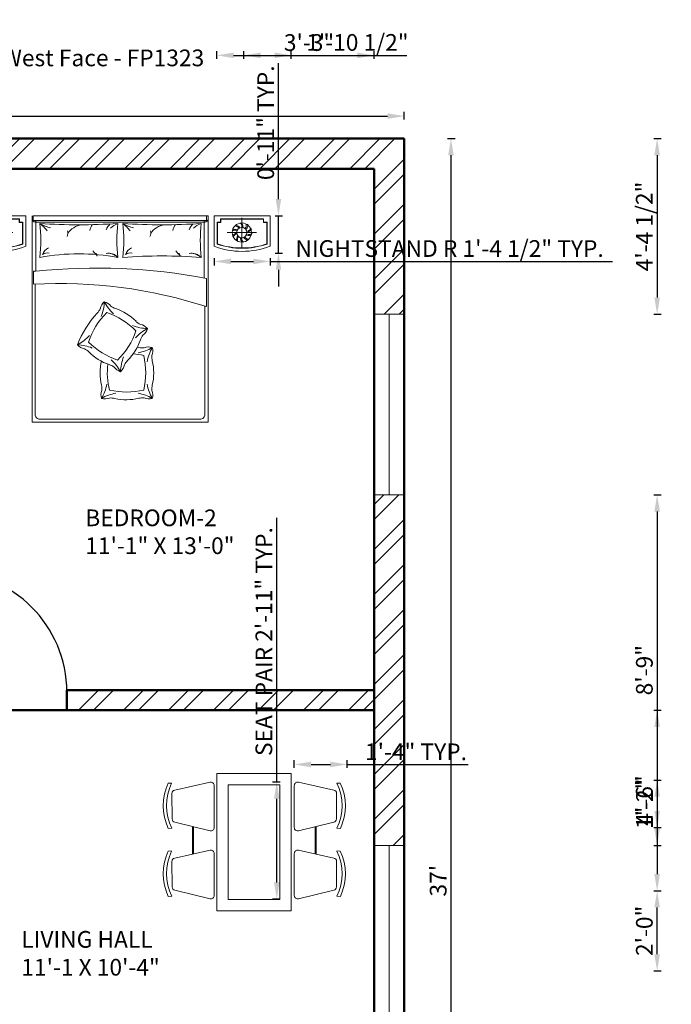
# Model space of a CAD drawing. Units: inches. Extents: x -83 to 371, y -457 to 76.
# Tile 4 of 4: x 176 to 371, y -243 to 51. Entities that reach past the tile are written whole.
import ezdxf

# ---------------------------------------------------------------- set-up
doc = ezdxf.new("R2010")
doc.units = ezdxf.units.IN
for name, color, linetype, lineweight in [('A-ANNO-DIMS', 2, 'Continuous', 18), ('A-ANNO-TEXT', 7, 'Continuous', 25), ('A-AREA-IDEN', 7, 'Continuous', 25), ('A-DOOR', 3, 'Continuous', 25), ('A-GLAZ', 4, 'Continuous', 18), ('A-WALL', 7, 'Continuous', 50), ('A-WALL-PATT', 252, 'Continuous', 13), ('furn', 28, 'Continuous', 18)]:
    doc.layers.add(name, color=color, linetype=linetype, lineweight=lineweight)
doc.styles.get("Standard").update_dxf_attribs({"font": 'arial.ttf'})
doc.dimstyles.new('ISO-25', dxfattribs={"dimtxt": 5, "dimasz": 5, "dimexe": 1.25, "dimexo": 0.625, "dimtad": 1, "dimlunit": 3, "dimtxsty": 'Standard', "dimcen": 2.5, "dimadec": 0, "dimazin": 0, "dimtfac": 1, "dimtmove": 0, "dimatfit": 3, "dimfxl": 1, "dimfxlon": 1, "dimarcsym": 0})

# ---------------------------------------------------------------- blocks, each defined once
blk = doc.blocks.new('*U4')
for p, q in [((0, 0), (0, -6)), ((40, 0), (40, -6))]:
    blk.add_line(p, q)
blk.add_lwpolyline([(0, 0), (0, 40), (1.75, 40), (1.75, 0)], close=True)
blk.add_arc((0, 0), 40, 0, 90)
blk = doc.blocks.new('*D8')
at = {"layer": 'A-ANNO-DIMS', "color": 0, "lineweight": -2, "transparency": 16777216}
for p, q in [((2.97, 21.4), (2.97, 23.65)), ((290.97, 21.4), (290.97, 23.65)), ((7.97, 22.4), (285.97, 22.4))]:
    blk.add_line(p, q, dxfattribs=at)
at = {"layer": 'A-ANNO-DIMS', "color": 0, "transparency": 16777216}
for points in [[(7.97, 23.23), (7.97, 21.56), (2.97, 22.4)], [(285.97, 23.23), (285.97, 21.56), (290.97, 22.4)]]:
    blk.add_solid(points, dxfattribs=at)
at = {"layer": 'Defpoints', "color": 0, "transparency": 16777216}
for p in [(290.97, 22.4), (2.97, 15.68), (290.97, 15.68)]:
    blk.add_point(p, dxfattribs=at)
at = {"layer": 'A-ANNO-DIMS', "color": 0, "transparency": 16777216, "insert": (146.97, 25.53), "char_height": 5, "attachment_point": 5}
blk.add_mtext("24'", dxfattribs=at)
blk = doc.blocks.new('*D9')
at = {"layer": 'A-ANNO-DIMS', "color": 0, "lineweight": -2, "transparency": 16777216}
for p, q in [((303.95, 15.68), (306.2, 15.68)), ((304.95, 10.68), (304.95, -423.32)), ((303.95, -428.32), (306.2, -428.32))]:
    blk.add_line(p, q, dxfattribs=at)
at = {"layer": 'A-ANNO-DIMS', "color": 0, "transparency": 16777216}
for points in [[(304.12, 10.68), (305.78, 10.68), (304.95, 15.68)], [(304.12, -423.32), (305.78, -423.32), (304.95, -428.32)]]:
    blk.add_solid(points, dxfattribs=at)
at = {"layer": 'Defpoints', "color": 0, "transparency": 16777216}
for p in [(295.93, 15.68), (290.97, -428.32), (304.95, -428.32)]:
    blk.add_point(p, dxfattribs=at)
at = {"layer": 'A-ANNO-DIMS', "color": 0, "transparency": 16777216, "insert": (301.77, -206.32), "char_height": 5, "attachment_point": 5, "rotation": 90}
blk.add_mtext("37'", dxfattribs=at)
blk = doc.blocks.new('BED-DOUBLE')
for p, q in [((0.91, 59.91), (51.75, 59.91)), ((1.17, 60.37), (1.17, 45.16)), ((51.46, 60.37), (51.46, 43.19))]:
    blk.add_line(p, q)
for points in [[(0, 61.8), (0, 0), (52.66, 0), (52.66, 61.8)], [(52.17, 61.8), (52.17, 60.37), (0.3, 60.37), (0.3, 61.8), (52.66, 61.8)]]:
    blk.add_lwpolyline(points)
for points in [[(2.33, 49.32, 0.058596), (2.33, 59.5, 0.036889), (25.64, 59.5, 0.052163), (25.64, 49.32, 0.093111)], [(27.16, 49.32, 0.058596), (27.16, 59.5, 0.036648), (50.62, 59.5, 0.052163), (50.62, 49.32, 0.036967)], [(0.46, 45.16), (1.17, 45.16, -0.072944), (52.17, 43.04), (52.17, 34.6, 0.092568), (0.46, 41.29)]]:
    blk.add_lwpolyline(points, format="xyb", close=True)
for points in [[(0.91, 41.32), (0.91, 2.43, 0.414214), (2.43, 0.91), (50.23, 0.91, 0.414214), (51.75, 2.43), (51.75, 34.75)], [(20.68, 31.62, 0.091296), (21.61, 36.08, 0.091296), (24.41, 32.49, 0.091296)], [(16.91, 24, 0.111006), (25.6, 18.59, 0.119549), (31.09, 27.39, 0.107813), (22.42, 32.82)], [(22.37, 32.81, 0.121865), (16.91, 24, 0.121865)], [(26.47, 15.11, 0.159461), (27.65, 17.2, -0.076283), (28.59, 18.51, 0.115075), (32.41, 24.64, -0.076283), (33.17, 26.05, 0.159461), (34.52, 28.03)], [(30.07, 28.97, 0.091296), (34.52, 28.03, 0.091296), (30.93, 25.24, 0.091296)], [(18.01, 22.22, 0.091296), (13.56, 23.16, 0.091296), (17.15, 25.96, 0.091296)], [(31.71, 20.79, 0.091296), (35.99, 22.35, 0.091296), (34.42, 18.08, 0.091296)], [(35.99, 7.13, 0.159461), (35.88, 9.53, -0.076283), (35.99, 11.13, 0.115075), (35.99, 18.36, -0.076283), (35.88, 19.96, 0.159461), (35.99, 22.35)], [(23.17, 9.62, 0.111006), (33.41, 9.63, 0.119549), (33.41, 19.99, 0.033212), (30.26, 20.47)], [(27.4, 19.57, 0.091296), (26.47, 15.11, 0.091296), (23.67, 18.7)], [(25.05, 8.69, 0.091296), (20.77, 7.13, 0.091296), (22.34, 11.41, 0.091296)], [(34.42, 11.41, 0.091296), (35.99, 7.13, 0.091296), (31.71, 8.69)]]:
    blk.add_lwpolyline(points, format="xyb")
for centre, radius, start, end in [((0.91, 60.83), 0.913, 180, 270), ((7.74, 68), 10.08, 237.5379, 257.5233), ((-5.29, 49.98), 12.19, 36.4935, 51.2792), ((15.48, 53.46), 5.64, 96.6849, 148.3182), ((21.18, 56.67), 3.96, 141.8174, 169.8987), ((26.19, 56.11), 4.26, 130.5354, 160.3558), ((28.84, 52.52), 7.67, 114.6457, 134.1585), ((19.53, 49.98), 12.19, 36.4935, 51.2792), ((32.57, 68), 10.08, 237.5379, 257.5233), ((40.3, 53.46), 5.64, 96.6849, 148.3182), ((46.01, 56.67), 3.96, 141.8174, 169.8987), ((51.01, 56.11), 4.26, 130.5354, 160.3558), ((53.67, 52.52), 7.67, 114.6457, 134.1585), ((51.75, 60.83), 0.913, 270, 0), ((8.15, 56.6), 2.53, 335.8927, 16.1192), ((32.98, 56.6), 2.53, 335.8927, 16.1192), ((6.34, 49.09), 3.38, 114.2916, 160.9896), ((4.59, 48.38), 2.31, 76.4823, 128.5563), ((9.19, 42.25), 12.71, 36.2085, 45.0849), ((18.6, 49.75), 0.853, 353.7543, 77.2187), ((22.67, 46.41), 4.16, 44.406, 96.8342), ((23.45, 47.86), 2.64, 33.6349, 90.8456), ((31.17, 49.09), 3.38, 114.2916, 160.9896), ((29.41, 48.38), 2.31, 76.4823, 128.5563), ((34.02, 42.25), 12.71, 36.2085, 45.0849), ((43.42, 49.75), 0.853, 353.7543, 77.2187), ((47.5, 46.41), 4.16, 44.406, 96.8342), ((48.27, 47.86), 2.64, 33.6349, 90.8456), ((24.21, 33.23), 3.86, 132.4658, 168.7065), ((20.58, 32.5), 3.72, 37.2937, 74.0973), ((44.41, 10.55), 33.33, 138.3818, 157.7644), ((15.72, 36.39), 5.29, 315.5854, 333.0343), ((26.71, 38.99), 5.29, 233.2983, 250.7472), ((19.89, 18.93), 15.91, 45.1307, 71.3884), ((34.79, 33.99), 5.29, 225.7718, 243.2208), ((31.77, 25.77), 3.56, 39.4726, 79.6505), ((16.39, 25.78), 3.86, 222.6522, 258.8929), ((13.27, 17.27), 5.29, 45.7718, 63.2208), ((28.18, 32.33), 15.91, 225.1307, 251.3884), ((28.38, 6.89), 15.91, 77.0576, 78.7033), ((33.07, 27.55), 5.29, 257.6988, 275.1477), ((34.85, 18.98), 3.56, 71.3996, 111.5774), ((36.26, 14.74), 15.91, 166.8711, 193.1289), ((44.1, 14.85), 21.58, 173.1956, 194.0284), ((21.36, 12.27), 5.29, 53.2983, 70.7472), ((27.96, 19.27), 4.41, 218.7754, 250.3571), ((24.48, 8.17), 3.86, 159.3666, 195.6073), ((15.61, 9.99), 5.29, 355.0387, 12.4877), ((21.79, 10.85), 3.86, 254.5791, 290.8198), ((23.64, 1.98), 5.29, 77.6988, 95.1477), ((28.33, 22.65), 15.91, 257.0576, 283.3153), ((33.15, 2.01), 5.29, 85.2252, 102.6741), ((35.05, 11.45), 4.41, 250.7023, 282.284)]:
    blk.add_arc(centre, radius, start, end)
blk = doc.blocks.new('NIGHTSTAND-L')
for p, q in [((8.46, 1.22), (8.46, 10)), ((4.07, 5.61), (12.85, 5.61))]:
    blk.add_line(p, q)
blk.add_lwpolyline([(0, 1.52), (0, 10.65), (16.74, 10.65), (16.74, 1.52, -0.181818)], format="xyb", close=True)
for points in [[(1.92, 9.74), (1.92, 8.74), (0.91, 8.74)], [(2.01, 9.74), (2.01, 8.65), (0.91, 8.65)], [(1.92, 9.74), (14.83, 9.74)], [(1.92, 9.65), (14.83, 9.65)], [(14.73, 9.74), (14.73, 8.65), (15.83, 8.65)], [(14.83, 9.74), (14.83, 8.74), (15.83, 8.74)]]:
    blk.add_lwpolyline(points)
for points in [[(15.83, 8.74), (15.83, 2.16, -0.167087), (0.91, 2.16), (0.91, 8.74)], [(15.74, 8.74), (15.74, 2.22, -0.165559), (1, 2.22), (1, 8.74)]]:
    blk.add_lwpolyline(points, format="xyb")
for radius in [2.87, 1.55]:
    blk.add_circle((8.46, 5.61), radius)
for centre, radius, start, end in [((7.4, 7.5), 1.84, 208.17, 254.4897), ((7.28, 7.36), 1.41, 196.3002, 256.538), ((8.71, 7.76), 1.84, 172.17, 218.4897), ((8.53, 7.72), 1.41, 160.3002, 220.538), ((9.93, 7.2), 1.84, 136.17, 182.4897), ((9.76, 7.27), 1.41, 124.3002, 184.538), ((10.58, 6.04), 1.84, 100.17, 146.4897), ((10.49, 6.19), 1.41, 88.3002, 148.538), ((10.42, 4.71), 1.84, 64.17, 110.4897), ((10.44, 4.89), 1.41, 52.3002, 112.538), ((6.48, 6.34), 1.41, 232.3002, 292.538), ((6.49, 6.52), 1.84, 244.17, 290.4897), ((6.43, 5.03), 1.41, 268.3002, 328.538), ((6.34, 5.19), 1.84, 280.17, 326.4897), ((7.16, 3.95), 1.41, 304.3002, 4.538), ((6.99, 4.02), 1.84, 316.17, 2.4897), ((8.38, 3.51), 1.41, 340.3002, 40.538), ((8.2, 3.47), 1.84, 352.17, 38.4897), ((9.64, 3.86), 1.41, 16.3002, 76.538), ((9.52, 3.73), 1.84, 28.17, 74.4897)]:
    blk.add_arc(centre, radius, start, end)
blk = doc.blocks.new('NIGHTSTAND-R')
for p, q in [((8.28, 1.22), (8.28, 10)), ((12.67, 5.61), (3.89, 5.61))]:
    blk.add_line(p, q)
blk.add_lwpolyline([(16.74, 1.52), (16.74, 10.65), (0, 10.65), (0, 1.52, 0.181818)], format="xyb", close=True)
for points in [[(1.92, 9.74), (1.92, 8.74), (0.91, 8.74)], [(2.01, 9.74), (2.01, 8.65), (0.91, 8.65)], [(14.82, 9.74), (1.92, 9.74)], [(14.82, 9.65), (1.92, 9.65)], [(14.73, 9.74), (14.73, 8.65), (15.83, 8.65)], [(14.82, 9.74), (14.82, 8.74), (15.83, 8.74)]]:
    blk.add_lwpolyline(points)
for points in [[(0.91, 8.74), (0.91, 2.16, 0.167087), (15.83, 2.16), (15.83, 8.74)], [(1, 8.74), (1, 2.22, 0.165559), (15.74, 2.22), (15.74, 8.74)]]:
    blk.add_lwpolyline(points, format="xyb")
for radius in [2.87, 1.55]:
    blk.add_circle((8.28, 5.61), radius)
for centre, radius, start, end in [((6.3, 4.89), 1.41, 67.462, 127.6998), ((6.32, 4.7), 1.84, 69.5103, 115.83), ((6.26, 6.19), 1.41, 31.462, 91.6998), ((6.16, 6.03), 1.84, 33.5103, 79.83), ((6.99, 7.27), 1.41, 355.462, 55.6998), ((6.82, 7.2), 1.84, 357.5103, 43.83), ((8.21, 7.72), 1.41, 319.462, 19.6998), ((8.24, 7.84), 1.84, 321.5103, 7.83), ((9.67, 7.44), 1.41, 283.462, 343.6998), ((9.55, 7.58), 1.84, 285.5103, 331.83), ((7.23, 3.72), 1.84, 105.5103, 151.83), ((7.11, 3.86), 1.41, 103.462, 163.6998), ((8.54, 3.46), 1.84, 141.5103, 187.83), ((8.36, 3.5), 1.41, 139.462, 199.6998), ((9.75, 4.02), 1.84, 177.5103, 223.83), ((9.58, 3.95), 1.41, 175.462, 235.6998), ((10.41, 5.19), 1.84, 213.5103, 259.83), ((10.31, 5.03), 1.41, 211.462, 271.6998), ((10.46, 6.59), 1.84, 249.5103, 295.83), ((10.48, 6.41), 1.41, 247.462, 307.6998)]:
    blk.add_arc(centre, radius, start, end)
blk = doc.blocks.new('DINING-SEAT-PAIR')
for p, q in [((6.2, 21.56), (6.2, 13.49)), ((6.54, 21.64), (6.54, 13.41))]:
    blk.add_line(p, q)
for points in [[(12.6, 23.92), (12.66, 31.56, 0.354445), (11.85, 32.57), (1.25, 34.9, 0.479008), (0, 33.9), (0, 21.36, 0.486085), (1.27, 20.36), (11.81, 22.93, 0.343643)], [(12.6, 3.59), (12.66, 11.23, 0.354445), (11.85, 12.24), (1.25, 14.57, 0.479008), (0, 13.57), (0, 1.03, 0.486085), (1.27, 0.03), (11.81, 2.6, 0.343643)]]:
    blk.add_lwpolyline(points, format="xyb", close=True)
for points in [[(12.77, 34.67), (13.75, 34.63, -0.22351), (13.78, 21.09), (12.74, 21.13, 0.225963), (12.77, 34.63, -0.224559)], [(12.77, 14.34), (13.75, 14.3, -0.22351), (13.78, 0.77), (12.74, 0.8, 0.225963), (12.77, 14.3, -0.224559)]]:
    blk.add_lwpolyline(points, format="xyb")
blk = doc.blocks.new('WIN-54IN')
blk.add_line((4.5, 54), (4.5, 0))
blk.add_lwpolyline([(0, 54), (9, 54), (9, 0), (0, 0)], close=True)
blk = doc.blocks.new('*D26')
at = {"layer": 'A-ANNO-DIMS', "color": 0, "lineweight": -2, "transparency": 16777216}
for p, q in [((234.07, -20.07), (234.07, -22.32)), ((250.81, -20.07), (250.81, -22.32)), ((239.07, -21.07), (245.81, -21.07)), ((250.81, -21.07), (353.27, -21.07))]:
    blk.add_line(p, q, dxfattribs=at)
at = {"layer": 'A-ANNO-DIMS', "color": 0, "transparency": 16777216}
for points in [[(239.07, -20.23), (239.07, -21.9), (234.07, -21.07)], [(245.81, -20.23), (245.81, -21.9), (250.81, -21.07)]]:
    blk.add_solid(points, dxfattribs=at)
at = {"layer": 'Defpoints', "color": 0, "transparency": 16777216}
for p in [(234.07, -18.56), (250.81, -18.56), (250.81, -21.07)]:
    blk.add_point(p, dxfattribs=at)
at = {"layer": 'A-ANNO-DIMS', "color": 0, "transparency": 16777216, "insert": (304.54, -17.86), "char_height": 5, "attachment_point": 5}
blk.add_mtext('NIGHTSTAND R 1\'-4 1/2" TYP.', dxfattribs=at)
blk = doc.blocks.new('*D27')
at = {"layer": 'A-ANNO-DIMS', "color": 0, "lineweight": -2, "transparency": 16777216}
for p, q in [((253.32, -2.4), (253.32, 38.22)), ((252.32, -7.4), (254.57, -7.4)), ((253.32, -18.56), (253.32, -7.4)), ((252.32, -18.56), (254.57, -18.56)), ((253.32, -23.56), (253.32, -28.56))]:
    blk.add_line(p, q, dxfattribs=at)
at = {"layer": 'A-ANNO-DIMS', "color": 0, "transparency": 16777216}
for points in [[(252.49, -2.4), (254.15, -2.4), (253.32, -7.4)], [(252.49, -23.56), (254.15, -23.56), (253.32, -18.56)]]:
    blk.add_solid(points, dxfattribs=at)
at = {"layer": 'Defpoints', "color": 0, "transparency": 16777216}
for p in [(250.81, -7.4), (253.32, -7.4), (250.81, -18.56)]:
    blk.add_point(p, dxfattribs=at)
at = {"layer": 'A-ANNO-DIMS', "color": 0, "transparency": 16777216, "insert": (250.14, 20.41), "char_height": 5, "attachment_point": 5, "rotation": 90}
blk.add_mtext('0\'-11" TYP.', dxfattribs=at)
blk = doc.blocks.new('*D28')
at = {"layer": 'A-ANNO-DIMS', "color": 0, "lineweight": -2, "transparency": 16777216}
for p, q in [((252.81, -176.8), (252.81, -97.79)), ((253.81, -176.8), (251.56, -176.8)), ((252.81, -206.81), (252.81, -181.8)), ((253.81, -211.81), (251.56, -211.81))]:
    blk.add_line(p, q, dxfattribs=at)
at = {"layer": 'A-ANNO-DIMS', "color": 0, "transparency": 16777216}
for points in [[(251.98, -181.8), (253.64, -181.8), (252.81, -176.8)], [(251.98, -206.81), (253.64, -206.81), (252.81, -211.81)]]:
    blk.add_solid(points, dxfattribs=at)
at = {"layer": 'Defpoints', "color": 0, "transparency": 16777216}
for p in [(252.81, -176.8), (258.06, -176.8), (258.06, -211.81)]:
    blk.add_point(p, dxfattribs=at)
at = {"layer": 'A-ANNO-DIMS', "color": 0, "transparency": 16777216, "insert": (249.6, -134.79), "char_height": 5, "attachment_point": 5, "rotation": 90}
blk.add_mtext('SEAT PAIR 2\'-11" TYP.', dxfattribs=at)
blk = doc.blocks.new('*D29')
at = {"layer": 'A-ANNO-DIMS', "color": 0, "lineweight": -2, "transparency": 16777216}
for p, q in [((258.06, -172.55), (258.06, -170.3)), ((273.85, -172.55), (273.85, -170.3)), ((263.06, -171.55), (268.85, -171.55)), ((273.85, -171.55), (310.11, -171.55))]:
    blk.add_line(p, q, dxfattribs=at)
at = {"layer": 'A-ANNO-DIMS', "color": 0, "transparency": 16777216}
for points in [[(263.06, -170.72), (263.06, -172.38), (258.06, -171.55)], [(268.85, -170.72), (268.85, -172.38), (273.85, -171.55)]]:
    blk.add_solid(points, dxfattribs=at)
at = {"layer": 'Defpoints', "color": 0, "transparency": 16777216}
for p in [(273.85, -171.55), (258.06, -176.8), (273.85, -176.8)]:
    blk.add_point(p, dxfattribs=at)
at = {"layer": 'A-ANNO-DIMS', "color": 0, "transparency": 16777216, "insert": (294.48, -168.41), "char_height": 5, "attachment_point": 5}
blk.add_mtext('1\'-4" TYP.', dxfattribs=at)
blk = doc.blocks.new('*D42')
at = {"layer": 'A-ANNO-DIMS', "color": 0, "lineweight": -2, "transparency": 16777216}
for p, q in [((365.66, 15.68), (367.91, 15.68)), ((366.66, 10.68), (366.66, -31.89)), ((365.66, -36.89), (367.91, -36.89))]:
    blk.add_line(p, q, dxfattribs=at)
at = {"layer": 'A-ANNO-DIMS', "color": 0, "transparency": 16777216}
for points in [[(365.83, 10.68), (367.49, 10.68), (366.66, 15.68)], [(365.83, -31.89), (367.49, -31.89), (366.66, -36.89)]]:
    blk.add_solid(points, dxfattribs=at)
at = {"layer": 'Defpoints', "color": 0, "transparency": 16777216}
for p in [(290.97, 15.68), (290.97, -36.89), (366.66, -36.89)]:
    blk.add_point(p, dxfattribs=at)
at = {"layer": 'A-ANNO-DIMS', "color": 0, "transparency": 16777216, "insert": (363.45, -10.61), "char_height": 5, "attachment_point": 5, "rotation": 90}
blk.add_mtext('4\'-4 1/2"', dxfattribs=at)
blk = doc.blocks.new('*D43')
at = {"layer": 'A-ANNO-DIMS', "color": 0, "lineweight": -2, "transparency": 16777216}
for p, q in [((365.66, -90.89), (367.91, -90.89)), ((366.66, -95.89), (366.66, -190.79)), ((365.66, -195.79), (367.91, -195.79))]:
    blk.add_line(p, q, dxfattribs=at)
at = {"layer": 'A-ANNO-DIMS', "color": 0, "transparency": 16777216}
for points in [[(365.83, -95.89), (367.49, -95.89), (366.66, -90.89)], [(365.83, -190.79), (367.49, -190.79), (366.66, -195.79)]]:
    blk.add_solid(points, dxfattribs=at)
at = {"layer": 'Defpoints', "color": 0, "transparency": 16777216}
for p in [(290.97, -90.89), (290.97, -195.79), (366.66, -195.79)]:
    blk.add_point(p, dxfattribs=at)
at = {"layer": 'A-ANNO-DIMS', "color": 0, "transparency": 16777216, "insert": (363.48, -143.34), "char_height": 5, "attachment_point": 5, "rotation": 90}
blk.add_mtext('8\'-9"', dxfattribs=at)
blk = doc.blocks.new('*D48')
at = {"layer": 'A-ANNO-DIMS', "color": 0, "lineweight": -2, "transparency": 16777216}
for p, q in [((242.97, 39.58), (242.97, 41.83)), ((281.97, 39.58), (281.97, 41.83)), ((247.97, 40.58), (276.97, 40.58))]:
    blk.add_line(p, q, dxfattribs=at)
at = {"layer": 'A-ANNO-DIMS', "color": 0, "transparency": 16777216}
for points in [[(247.97, 41.41), (247.97, 39.74), (242.97, 40.58)], [(276.97, 41.41), (276.97, 39.74), (281.97, 40.58)]]:
    blk.add_solid(points, dxfattribs=at)
at = {"layer": 'Defpoints', "color": 0, "transparency": 16777216}
for p in [(281.97, 40.58), (242.97, -266.56), (281.97, -266.56)]:
    blk.add_point(p, dxfattribs=at)
at = {"layer": 'A-ANNO-DIMS', "color": 0, "transparency": 16777216, "insert": (262.47, 43.75), "char_height": 5, "attachment_point": 5}
blk.add_mtext('3\'-3"', dxfattribs=at)
blk = doc.blocks.new('*D56')
at = {"layer": 'A-ANNO-DIMS', "color": 0, "lineweight": -2, "transparency": 16777216}
for p, q in [((365.66, -209.32), (367.91, -209.32)), ((366.66, -228.32), (366.66, -214.32)), ((365.66, -233.32), (367.91, -233.32))]:
    blk.add_line(p, q, dxfattribs=at)
at = {"layer": 'A-ANNO-DIMS', "color": 0, "transparency": 16777216}
for points in [[(365.83, -214.32), (367.49, -214.32), (366.66, -209.32)], [(365.83, -228.32), (367.49, -228.32), (366.66, -233.32)]]:
    blk.add_solid(points, dxfattribs=at)
at = {"layer": 'Defpoints', "color": 0, "transparency": 16777216}
for p in [(103.87, -209.32), (366.66, -209.32), (103.87, -233.32)]:
    blk.add_point(p, dxfattribs=at)
at = {"layer": 'A-ANNO-DIMS', "color": 0, "transparency": 16777216, "insert": (363.48, -221.32), "char_height": 5, "attachment_point": 5, "rotation": 90}
blk.add_mtext('2\'-0"', dxfattribs=at)
blk = doc.blocks.new('*D57')
at = {"layer": 'A-ANNO-DIMS', "color": 0, "lineweight": -2, "transparency": 16777216}
for p, q in [((365.66, -155.32), (367.91, -155.32)), ((366.66, -160.32), (366.66, -204.32)), ((365.66, -209.32), (367.91, -209.32))]:
    blk.add_line(p, q, dxfattribs=at)
at = {"layer": 'A-ANNO-DIMS', "color": 0, "transparency": 16777216}
for points in [[(365.83, -160.32), (367.49, -160.32), (366.66, -155.32)], [(365.83, -204.32), (367.49, -204.32), (366.66, -209.32)]]:
    blk.add_solid(points, dxfattribs=at)
at = {"layer": 'Defpoints', "color": 0, "transparency": 16777216}
for p in [(35.97, -155.32), (35.97, -209.32), (366.66, -209.32)]:
    blk.add_point(p, dxfattribs=at)
at = {"layer": 'A-ANNO-DIMS', "color": 0, "transparency": 16777216, "insert": (363.48, -182.32), "char_height": 5, "attachment_point": 5, "rotation": 90}
blk.add_mtext('4\'-6"', dxfattribs=at)
blk = doc.blocks.new('*D60')
at = {"layer": 'A-ANNO-DIMS', "color": 0, "lineweight": -2, "transparency": 16777216}
for p, q in [((365.66, -176.2), (367.91, -176.2)), ((366.66, -181.2), (366.66, -185.42)), ((365.66, -190.42), (367.91, -190.42))]:
    blk.add_line(p, q, dxfattribs=at)
at = {"layer": 'A-ANNO-DIMS', "color": 0, "transparency": 16777216}
for points in [[(365.83, -181.2), (367.49, -181.2), (366.66, -176.2)], [(365.83, -185.42), (367.49, -185.42), (366.66, -190.42)]]:
    blk.add_solid(points, dxfattribs=at)
at = {"layer": 'Defpoints', "color": 0, "transparency": 16777216}
for p in [(31.73, -176.2), (31.73, -190.42), (366.66, -190.42)]:
    blk.add_point(p, dxfattribs=at)
at = {"layer": 'A-ANNO-DIMS', "color": 0, "transparency": 16777216, "insert": (363.52, -183.31), "char_height": 5, "attachment_point": 5, "rotation": 90}
blk.add_mtext('1\'-2"', dxfattribs=at)
blk = doc.blocks.new('*D61')
at = {"layer": 'A-ANNO-DIMS', "color": 0, "lineweight": -2, "transparency": 16777216}
for p, q in [((234.88, 39.58), (234.88, 41.83)), ((257.14, 39.58), (257.14, 41.83)), ((239.88, 40.58), (252.14, 40.58)), ((257.14, 40.58), (291.75, 40.58))]:
    blk.add_line(p, q, dxfattribs=at)
at = {"layer": 'A-ANNO-DIMS', "color": 0, "transparency": 16777216}
for points in [[(239.88, 41.41), (239.88, 39.74), (234.88, 40.58)], [(252.14, 41.41), (252.14, 39.74), (257.14, 40.58)]]:
    blk.add_solid(points, dxfattribs=at)
at = {"layer": 'Defpoints', "color": 0, "transparency": 16777216}
for p in [(257.14, 40.58), (234.88, -174.24), (257.14, -174.24)]:
    blk.add_point(p, dxfattribs=at)
at = {"layer": 'A-ANNO-DIMS', "color": 0, "transparency": 16777216, "insert": (276.95, 43.79), "char_height": 5, "attachment_point": 5}
blk.add_mtext('1\'-10 1/2"', dxfattribs=at)
blk = doc.blocks.new('*D62')
at = {"layer": 'A-ANNO-DIMS', "color": 0, "lineweight": -2, "transparency": 16777216}
for p, q in [((-71.36, -174.24), (-73.61, -174.24)), ((-72.36, -179.24), (-72.36, -210.33)), ((-71.36, -215.33), (-73.61, -215.33))]:
    blk.add_line(p, q, dxfattribs=at)
at = {"layer": 'A-ANNO-DIMS', "color": 0, "transparency": 16777216}
for points in [[(-73.19, -179.24), (-71.52, -179.24), (-72.36, -174.24)], [(-73.19, -210.33), (-71.52, -210.33), (-72.36, -215.33)]]:
    blk.add_solid(points, dxfattribs=at)
at = {"layer": 'Defpoints', "color": 0, "transparency": 16777216}
for p in [(234.88, -174.24), (-72.36, -215.33), (234.88, -215.33)]:
    blk.add_point(p, dxfattribs=at)
at = {"layer": 'A-ANNO-DIMS', "color": 0, "transparency": 16777216, "insert": (-75.54, -194.79), "char_height": 5, "attachment_point": 5, "rotation": 90}
blk.add_mtext('3\'-5"', dxfattribs=at)

msp = doc.modelspace()

# ---------------------------------------------------------------- hatches: boundary and pattern name
at = {"layer": 'A-WALL-PATT'}
h = msp.add_hatch(dxfattribs=at)
h.set_pattern_fill('ANSI32', color=256)
h.set_pattern_definition([(45, (-445.966, 5e-14), (-6.73519, 6.73519), []), (45, (-441.476, 5e-14), (-6.73519, 6.73519), [])])
h.paths.add_polyline_path([(147.969, -419.325), (11.969, -419.325), (11.969, -408.128), (2.969, -408.128), (2.969, -428.325), (147.969, -428.325)])
h.paths.add_polyline_path([(290.969, -408.128), (281.969, -408.128), (281.969, -419.325), (197.969, -419.325), (197.969, -428.325), (290.969, -428.325)])
h.paths.add_polyline_path([(203.969, -374.325), (207.969, -374.325), (207.969, -368.325), (203.969, -368.325), (203.969, -279.294), (197.969, -279.294), (197.969, -317.37), (194.142, -317.37), (194.142, -317.678), (194.142, -323.37), (197.969, -323.37), (197.969, -374.325), (197.969, -419.325), (203.969, -419.325)])
h.paths.add_polyline_path([(290.969, -249.793), (281.969, -249.793), (281.969, -390.128), (290.969, -390.128)])
h.paths.add_polyline_path([(149.969, -323.37), (157.969, -323.37), (157.969, -317.37), (149.969, -317.37), (149.969, -279.294), (143.969, -279.294), (143.969, -371.325), (140.142, -371.325), (140.142, -371.632), (140.142, -377.325), (143.969, -377.325), (149.969, -377.325)])
h.paths.add_polyline_path([(103.969, -371.325), (11.969, -371.325), (11.969, -377.325), (103.969, -377.325)])
h.paths.add_polyline_path([(11.969, -328.391), (3.855, -328.391), (3.855, -274.391), (11.969, -274.391), (11.969, -222.986), (2.969, -222.986), (2.969, -390.128), (11.969, -390.128)])
h.paths.add_polyline_path([(149.969, -233.325), (143.969, -233.325), (11.969, -233.325), (11.969, -239.325), (143.969, -239.325), (143.969, -243.294), (144.688, -243.294), (149.969, -243.294)])
h.paths.add_polyline_path([(11.969, -86.501), (2.969, -86.501), (2.969, -168.986), (11.969, -168.986)])
h.paths.add_polyline_path([(103.969, -149.325), (11.969, -149.325), (11.969, -155.325), (103.969, -155.325)])
h.paths.add_polyline_path([(149.969, 6.675), (143.969, 6.675), (143.969, -149.325), (139.969, -149.325), (139.969, -155.325), (153.969, -155.325), (153.969, -149.325), (149.969, -149.325)])
h.paths.add_polyline_path([(281.969, -149.325), (189.973, -149.325, -0.0041567), (189.978, -149.923), (189.978, -155.325), (281.969, -155.325)])
h.paths.add_polyline_path([(290.969, -90.886), (281.969, -90.886), (281.969, -195.793), (290.969, -195.793)])
h.paths.add_polyline_path([(290.969, 15.675), (2.969, 15.675), (2.969, -32.501), (11.969, -32.501), (11.969, 6.675), (281.969, 6.675), (281.969, -36.886), (290.969, -36.886)])

# ---------------------------------------------------------------- linework, layer by layer
at = {"layer": 'A-WALL'}
for p, q in [((2.969, 15.675), (290.969, 15.675)), ((290.969, 15.675), (290.969, -428.325)), ((11.969, 6.675), (281.969, 6.675)), ((281.969, 6.675), (281.969, -419.325)), ((189.969, -149.325), (189.969, -155.325)), ((189.969, -149.325), (281.969, -149.325)), ((11.969, -155.325), (281.969, -155.325))]:
    msp.add_line(p, q, dxfattribs=at)
at = {"layer": 'furn'}
for points in [[(257.142, -174.24), (234.884, -174.24), (234.884, -215.334), (257.142, -215.334)], [(253.718, -177.665), (238.308, -177.665), (238.308, -211.909), (253.718, -211.909)]]:
    msp.add_lwpolyline(points, close=True, dxfattribs=at)

# ---------------------------------------------------------------- block references
at = {"layer": 'A-DOOR', "xscale": 0.9002205977698526, "yscale": 0.9002205977698526, "zscale": 0.9002205977698526}
msp.add_blockref('*U4', (153.969, -149.923), dxfattribs=at)
at = {"layer": 'A-GLAZ'}
for p in [(281.969, -90.886), (281.969, -249.792)]:
    msp.add_blockref('WIN-54IN', p, dxfattribs=at)
at = {"layer": 'furn'}
for name, p in [('NIGHTSTAND-L', (161.006, -18.053)), ('BED-DOUBLE', (179.576, -69.19)), ('NIGHTSTAND-R', (234.066, -18.05)), ('DINING-SEAT-PAIR', (258.063, -211.769))]:
    msp.add_blockref(name, p, dxfattribs=at)
at = {"layer": 'furn', "extrusion": (0, 0, -1), "zscale": -1}
msp.add_blockref('DINING-SEAT-PAIR', (-234.106, -211.769), dxfattribs=at)

# ---------------------------------------------------------------- texts
at = {"layer": 'A-ANNO-TEXT', "insert": (75.772, 42.316), "char_height": 5, "attachment_point": 1}
msp.add_mtext_dynamic_manual_height_columns('24X37 (888 sq ft) House Plan - West Face - FP1323', width=296.42101, gutter_width=12.5, heights=[0], dxfattribs=at)
at = {"layer": 'A-AREA-IDEN', "char_height": 5, "attachment_point": 1}
for s, width, insert in [('BEDROOM-2\\P11\'-1" X 13\'-0"', 47.88686, (195.499, -95.273)), ('LIVING HALL\\P11\'-1 X 10\'-4"', 47.18704, (176.357, -221.372))]:
    msp.add_mtext_dynamic_manual_height_columns(s, width=width, gutter_width=12.5, heights=[0], dxfattribs=dict(at, insert=insert))

# ---------------------------------------------------------------- dimensions: what is measured, and where the dimension line sits
at = {"layer": 'A-ANNO-DIMS'}
for base, p1, p2, override, picture, middle in [((257.142, 40.575), (234.884, -174.24), (257.142, -174.24), {"dimdec": 1, "dimlfac": 1, "dimrnd": 0, "dimzin": 1, "dimdsep": 46, "dimlunit": 4, "dimfrac": 2}, '*D61', (276.946, 43.786)), ((281.969, 40.575), (242.969, -266.561), (281.969, -266.561), {"dimdec": 1, "dimlfac": 1, "dimrnd": 0, "dimzin": 1, "dimdsep": 46, "dimlunit": 4, "dimfrac": 2}, '*D48', (262.469, 43.755)), ((290.969, 22.396), (2.969, 15.675), (290.969, 15.675), {"dimclrd": 0, "dimclre": 0, "dimclrt": 0}, '*D8', (146.969, 25.531))]:
    dim = msp.add_linear_dim(base=base, p1=p1, p2=p2, dimstyle='ISO-25', override=override, dxfattribs=at)
    dim.commit()
    dim.dimension.update_dxf_attribs({"geometry": picture, "text_midpoint": middle})
for base, p1, p2, text, picture, middle in [((253.32, -7.395), (250.808, -18.557), (250.808, -7.395), '<> TYP.', '*D27', (250.142, 20.411)), ((252.811, -176.803), (258.063, -211.814), (258.063, -176.803), 'SEAT PAIR <> TYP.', '*D28', (249.601, -134.795))]:
    dim = msp.add_linear_dim(base=base, p1=p1, p2=p2, angle=90, text=text, dimstyle='ISO-25', override={"dimdec": 1, "dimlfac": 1, "dimrnd": 0, "dimzin": 1, "dimdsep": 46, "dimlunit": 4, "dimfrac": 2}, dxfattribs=at)
    dim.commit()
    dim.dimension.update_dxf_attribs({"geometry": picture, "text_midpoint": middle})
for base, p1, p2, override, picture, middle in [((304.949, -428.325), (295.93, 15.675), (290.969, -428.325), {"dimclrd": 0, "dimclre": 0, "dimclrt": 0}, '*D9', (301.769, -206.325)), ((366.659, -36.886), (290.969, 15.675), (290.969, -36.886), {"dimdec": 1, "dimlfac": 1, "dimrnd": 0, "dimzin": 1, "dimdsep": 46, "dimlunit": 4, "dimfrac": 2}, '*D42', (363.448, -10.606)), ((366.659, -195.793), (290.969, -90.886), (290.969, -195.793), {"dimdec": 1, "dimlfac": 1, "dimrnd": 0, "dimzin": 1, "dimdsep": 46, "dimlunit": 4, "dimfrac": 2}, '*D43', (363.481, -143.34)), ((366.659, -209.325), (35.969, -155.325), (35.969, -209.325), {"dimdec": 1, "dimlfac": 1, "dimrnd": 0, "dimzin": 1, "dimdsep": 46, "dimlunit": 4, "dimfrac": 2}, '*D57', (363.481, -182.325)), ((-72.358, -215.334), (234.884, -174.24), (234.884, -215.334), {"dimdec": 1, "dimlfac": 1, "dimrnd": 0, "dimzin": 1, "dimdsep": 46, "dimlunit": 4, "dimfrac": 2}, '*D62', (-75.538, -194.787)), ((366.659, -190.423), (31.729, -176.204), (31.729, -190.423), {"dimdec": 1, "dimlfac": 1, "dimrnd": 0, "dimzin": 1, "dimdsep": 46, "dimlunit": 4, "dimfrac": 2}, '*D60', (363.524, -183.314)), ((366.659, -209.325), (103.866, -233.325), (103.866, -209.325), {"dimdec": 1, "dimlfac": 1, "dimrnd": 0, "dimzin": 1, "dimdsep": 46, "dimlunit": 4, "dimfrac": 2}, '*D56', (363.481, -221.325))]:
    dim = msp.add_linear_dim(base=base, p1=p1, p2=p2, angle=90, dimstyle='ISO-25', override=override, dxfattribs=at)
    dim.commit()
    dim.dimension.update_dxf_attribs({"geometry": picture, "text_midpoint": middle})
for base, p1, p2, text, picture, middle in [((250.808, -21.068), (234.065, -18.557), (250.808, -18.557), 'NIGHTSTAND R <> TYP.', '*D26', (304.54, -17.858)), ((273.851, -171.551), (258.063, -176.803), (273.851, -176.803), '<> TYP.', '*D29', (294.48, -168.414))]:
    dim = msp.add_linear_dim(base=base, p1=p1, p2=p2, text=text, dimstyle='ISO-25', override={"dimdec": 1, "dimlfac": 1, "dimrnd": 0, "dimzin": 1, "dimdsep": 46, "dimlunit": 4, "dimfrac": 2}, dxfattribs=at)
    dim.commit()
    dim.dimension.update_dxf_attribs({"geometry": picture, "text_midpoint": middle})

doc.saveas('drawing.dxf')
